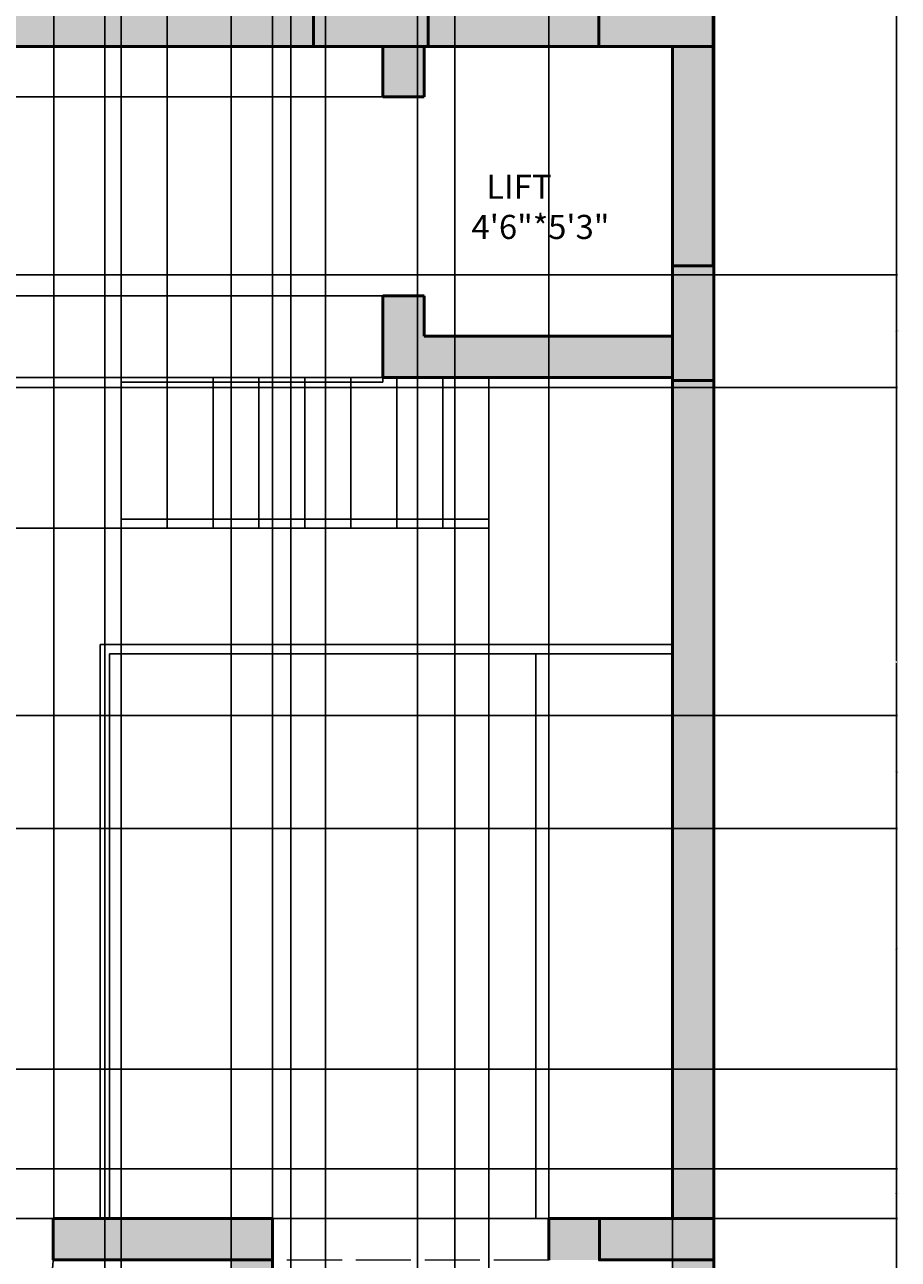
# Model space of a CAD drawing. Units: inches. Extents: x 2494 to 2908, y 1051 to 1885.
# Tile 5 of 7: x 2718 to 2908, y 1338 to 1607. Entities that reach past the tile are written whole.
import ezdxf

# ---------------------------------------------------------------- set-up
doc = ezdxf.new("R2010")
doc.units = ezdxf.units.IN
doc.linetypes.add('ACAD_ISO02W100', pattern=[15, 12, -3])
for name, color, linetype, lineweight in [('A-ANNO-DIMS', 2, 'Continuous', 18), ('A-AREA-IDEN', 130, 'Continuous', 18), ('A-COLS-PATT', 200, 'Continuous', 13), ('A-FLOR-HRAL', 140, 'Continuous', 25), ('A-FLOR-STRS', 7, 'Continuous', 25), ('A-WALL-OVHD', 140, 'ACAD_ISO02W100', 18), ('A-WALL-PATT', 140, 'Continuous', 13), ('COLUMN', 200, 'Continuous', 50), ('DOOR', 50, 'Continuous', 25), ('WALL', 140, 'Continuous', 50)]:
    doc.layers.add(name, color=color, linetype=linetype, lineweight=lineweight)
doc.styles.get("Standard").update_dxf_attribs({"font": 'arial.ttf'})
doc.dimstyles.get("Standard").update_dxf_attribs({"dimtxt": 0.18, "dimasz": 0.18, "dimexe": 0.18, "dimexo": 0.0625, "dimgap": 0.09, "dimtad": 0, "dimtih": 1, "dimtoh": 1, "dimdec": 4, "dimzin": 0, "dimdsep": 46, "dimtxsty": 'Standard', "dimcen": 0.09, "dimadec": 0, "dimazin": 0, "dimtfac": 1, "dimtdec": 4, "dimtofl": 0, "dimtmove": 0, "dimatfit": 3, "dimfxl": 1, "dimtolj": 1, "dimtzin": 0, "dimarcsym": 0})

# ---------------------------------------------------------------- blocks, each defined once
blk = doc.blocks.new('*U2')
for p, q in [((0, 0), (0, -6)), ((40, 0), (40, -6))]:
    blk.add_line(p, q)
blk.add_lwpolyline([(0, 0), (0, 40), (1.75, 40), (1.75, 0)], close=True)
blk.add_arc((0, 0), 40, 0, 90)
blk = doc.blocks.new('*D26')
at = {"layer": 'A-ANNO-DIMS', "color": 0, "lineweight": -2, "transparency": 16777216}
for p, q in [((2868.31, 1845.16), (2908.18, 1845.16)), ((2908, 1844.98), (2908, 1468.43)), ((2908, 1091.52), (2908, 1468.07)), ((2860.37, 1091.34), (2908.18, 1091.34))]:
    blk.add_line(p, q, dxfattribs=at)
at = {"layer": 'A-ANNO-DIMS', "color": 0, "lineweight": 100, "transparency": 16777216}
for points in [[(2907.97, 1844.98), (2908.03, 1844.98), (2908, 1845.16)], [(2907.97, 1091.52), (2908.03, 1091.52), (2908, 1091.34)]]:
    blk.add_solid(points, dxfattribs=at)
at = {"layer": 'Defpoints', "color": 0, "lineweight": 100, "transparency": 16777216}
for p in [(2868.25, 1845.16), (2908, 1845.16), (2860.3, 1091.34)]:
    blk.add_point(p, dxfattribs=at)
at = {"layer": 'A-ANNO-DIMS', "color": 0, "transparency": 16777216, "insert": (2908, 1468.25), "char_height": 0.18, "attachment_point": 5}
blk.add_mtext('\\A1;753.8', dxfattribs=at)
blk = doc.blocks.new('*D33')
at = {"layer": 'A-ANNO-DIMS', "color": 0, "lineweight": -2, "transparency": 16777216}
for p, q in [((2697.84, 1155.22), (2697.84, 1885.09)), ((2698.02, 1884.91), (2716.38, 1884.91)), ((2735.54, 1884.91), (2717.17, 1884.91)), ((2735.72, 1155.22), (2735.72, 1885.09))]:
    blk.add_line(p, q, dxfattribs=at)
at = {"layer": 'A-ANNO-DIMS', "color": 0, "lineweight": 100, "transparency": 16777216}
for points in [[(2698.02, 1884.94), (2698.02, 1884.88), (2697.84, 1884.91)], [(2735.54, 1884.94), (2735.54, 1884.88), (2735.72, 1884.91)]]:
    blk.add_solid(points, dxfattribs=at)
at = {"layer": 'Defpoints', "color": 0, "lineweight": 100, "transparency": 16777216}
for p in [(2735.72, 1884.91), (2697.84, 1155.16), (2735.72, 1155.16)]:
    blk.add_point(p, dxfattribs=at)
at = {"layer": 'A-ANNO-DIMS', "color": 0, "transparency": 16777216, "insert": (2716.78, 1884.91), "char_height": 0.18, "attachment_point": 5}
blk.add_mtext('\\A1;37.88', dxfattribs=at)
blk = doc.blocks.new('*D35')
at = {"layer": 'A-ANNO-DIMS', "color": 0, "lineweight": -2, "transparency": 16777216}
for p, q in [((2735.72, 1155.22), (2735.72, 1885.09)), ((2735.9, 1884.91), (2749.09, 1884.91)), ((2763.07, 1884.91), (2749.88, 1884.91)), ((2763.25, 1155.22), (2763.25, 1885.09))]:
    blk.add_line(p, q, dxfattribs=at)
at = {"layer": 'A-ANNO-DIMS', "color": 0, "lineweight": 100, "transparency": 16777216}
for points in [[(2735.9, 1884.94), (2735.9, 1884.88), (2735.72, 1884.91)], [(2763.07, 1884.94), (2763.07, 1884.88), (2763.25, 1884.91)]]:
    blk.add_solid(points, dxfattribs=at)
at = {"layer": 'Defpoints', "color": 0, "lineweight": 100, "transparency": 16777216}
for p in [(2763.25, 1884.91), (2735.72, 1155.16), (2763.25, 1155.16)]:
    blk.add_point(p, dxfattribs=at)
at = {"layer": 'A-ANNO-DIMS', "color": 0, "transparency": 16777216, "insert": (2749.49, 1884.91), "char_height": 0.18, "attachment_point": 5}
blk.add_mtext('\\A1;27.53', dxfattribs=at)
blk = doc.blocks.new('*D37')
at = {"layer": 'A-ANNO-DIMS', "color": 0, "lineweight": -2, "transparency": 16777216}
for p, q in [((2783.78, 1155.22), (2783.78, 1885.09)), ((2783.96, 1884.91), (2797.38, 1884.91)), ((2811.73, 1884.91), (2798.31, 1884.91)), ((2811.91, 1155.22), (2811.91, 1885.09))]:
    blk.add_line(p, q, dxfattribs=at)
at = {"layer": 'A-ANNO-DIMS', "color": 0, "lineweight": 100, "transparency": 16777216}
for points in [[(2783.96, 1884.94), (2783.96, 1884.88), (2783.78, 1884.91)], [(2811.73, 1884.94), (2811.73, 1884.88), (2811.91, 1884.91)]]:
    blk.add_solid(points, dxfattribs=at)
at = {"layer": 'Defpoints', "color": 0, "lineweight": 100, "transparency": 16777216}
for p in [(2811.91, 1884.91), (2783.78, 1155.16), (2811.91, 1155.16)]:
    blk.add_point(p, dxfattribs=at)
at = {"layer": 'A-ANNO-DIMS', "color": 0, "transparency": 16777216, "insert": (2797.85, 1884.91), "char_height": 0.18, "attachment_point": 5}
blk.add_mtext('\\A1;28.126', dxfattribs=at)
blk = doc.blocks.new('*D41')
at = {"layer": 'A-ANNO-DIMS', "color": 0, "lineweight": -2, "transparency": 16777216}
for p, q in [((2684.64, 1347.22), (2684.64, 1885.09)), ((2684.82, 1884.91), (2704.42, 1884.91)), ((2724.46, 1884.91), (2704.86, 1884.91)), ((2724.64, 1347.22), (2724.64, 1885.09))]:
    blk.add_line(p, q, dxfattribs=at)
at = {"layer": 'A-ANNO-DIMS', "color": 0, "lineweight": 100, "transparency": 16777216}
for points in [[(2684.82, 1884.94), (2684.82, 1884.88), (2684.64, 1884.91)], [(2724.46, 1884.94), (2724.46, 1884.88), (2724.64, 1884.91)]]:
    blk.add_solid(points, dxfattribs=at)
at = {"layer": 'Defpoints', "color": 0, "lineweight": 100, "transparency": 16777216}
for p in [(2724.64, 1884.91), (2684.64, 1347.16), (2724.64, 1347.16)]:
    blk.add_point(p, dxfattribs=at)
at = {"layer": 'A-ANNO-DIMS', "color": 0, "transparency": 16777216, "insert": (2704.64, 1884.91), "char_height": 0.18, "attachment_point": 5}
blk.add_mtext('\\A1;40', dxfattribs=at)
blk = doc.blocks.new('*D43')
at = {"layer": 'A-ANNO-DIMS', "color": 0, "lineweight": -2, "transparency": 16777216}
for p, q in [((2776.2, 1243.72), (2776.2, 1885.09)), ((2776.38, 1884.91), (2789.53, 1884.91)), ((2803.62, 1884.91), (2790.46, 1884.91)), ((2803.8, 1243.72), (2803.8, 1885.09))]:
    blk.add_line(p, q, dxfattribs=at)
at = {"layer": 'A-ANNO-DIMS', "color": 0, "lineweight": 100, "transparency": 16777216}
for points in [[(2776.38, 1884.94), (2776.38, 1884.88), (2776.2, 1884.91)], [(2803.62, 1884.94), (2803.62, 1884.88), (2803.8, 1884.91)]]:
    blk.add_solid(points, dxfattribs=at)
at = {"layer": 'Defpoints', "color": 0, "lineweight": 100, "transparency": 16777216}
for p in [(2803.8, 1884.91), (2776.2, 1243.66), (2803.8, 1243.66)]:
    blk.add_point(p, dxfattribs=at)
at = {"layer": 'A-ANNO-DIMS', "color": 0, "transparency": 16777216, "insert": (2790, 1884.91), "char_height": 0.18, "attachment_point": 5}
blk.add_mtext('\\A1;27.604', dxfattribs=at)
blk = doc.blocks.new('*D44')
at = {"layer": 'A-ANNO-DIMS', "color": 0, "lineweight": -2, "transparency": 16777216}
for p, q in [((2772.25, 1347.22), (2772.25, 1885.09)), ((2772.43, 1884.91), (2801.99, 1884.91)), ((2832.17, 1884.91), (2802.61, 1884.91)), ((2832.35, 1347.22), (2832.35, 1885.09))]:
    blk.add_line(p, q, dxfattribs=at)
at = {"layer": 'A-ANNO-DIMS', "color": 0, "lineweight": 100, "transparency": 16777216}
for points in [[(2772.43, 1884.94), (2772.43, 1884.88), (2772.25, 1884.91)], [(2832.17, 1884.94), (2832.17, 1884.88), (2832.35, 1884.91)]]:
    blk.add_solid(points, dxfattribs=at)
at = {"layer": 'Defpoints', "color": 0, "lineweight": 100, "transparency": 16777216}
for p in [(2832.35, 1884.91), (2772.25, 1347.16), (2832.35, 1347.16)]:
    blk.add_point(p, dxfattribs=at)
at = {"layer": 'A-ANNO-DIMS', "color": 0, "transparency": 16777216, "insert": (2802.3, 1884.91), "char_height": 0.18, "attachment_point": 5}
blk.add_mtext('\\A1;60.1', dxfattribs=at)
blk = doc.blocks.new('*D46')
at = {"layer": 'A-ANNO-DIMS', "color": 0, "lineweight": -2, "transparency": 16777216}
for p, q in [((2674.81, 1432.05), (2908.18, 1432.05)), ((2908, 1431.87), (2908, 1406.05)), ((2908, 1379.87), (2908, 1405.69)), ((2674.81, 1379.69), (2908.18, 1379.69))]:
    blk.add_line(p, q, dxfattribs=at)
at = {"layer": 'A-ANNO-DIMS', "color": 0, "lineweight": 100, "transparency": 16777216}
for points in [[(2907.97, 1431.87), (2908.03, 1431.87), (2908, 1432.05)], [(2907.97, 1379.87), (2908.03, 1379.87), (2908, 1379.69)]]:
    blk.add_solid(points, dxfattribs=at)
at = {"layer": 'Defpoints', "color": 0, "lineweight": 100, "transparency": 16777216}
for p in [(2674.75, 1432.05), (2908, 1432.05), (2674.75, 1379.69)]:
    blk.add_point(p, dxfattribs=at)
at = {"layer": 'A-ANNO-DIMS', "color": 0, "transparency": 16777216, "insert": (2908, 1405.87), "char_height": 0.18, "attachment_point": 5}
blk.add_mtext('\\A1;52.36', dxfattribs=at)
blk = doc.blocks.new('*D47')
at = {"layer": 'A-ANNO-DIMS', "color": 0, "lineweight": -2, "transparency": 16777216}
for p, q in [((2674.81, 1456.66), (2908.18, 1456.66)), ((2908, 1456.48), (2908, 1444.53)), ((2908, 1432.23), (2908, 1444.17)), ((2674.81, 1432.05), (2908.18, 1432.05))]:
    blk.add_line(p, q, dxfattribs=at)
at = {"layer": 'A-ANNO-DIMS', "color": 0, "lineweight": 100, "transparency": 16777216}
for points in [[(2907.97, 1456.48), (2908.03, 1456.48), (2908, 1456.66)], [(2907.97, 1432.23), (2908.03, 1432.23), (2908, 1432.05)]]:
    blk.add_solid(points, dxfattribs=at)
at = {"layer": 'Defpoints', "color": 0, "lineweight": 100, "transparency": 16777216}
for p in [(2674.75, 1456.66), (2908, 1456.66), (2674.75, 1432.05)]:
    blk.add_point(p, dxfattribs=at)
at = {"layer": 'A-ANNO-DIMS', "color": 0, "transparency": 16777216, "insert": (2908, 1444.35), "char_height": 0.18, "attachment_point": 5}
blk.add_mtext('\\A1;24.606', dxfattribs=at)
blk = doc.blocks.new('*D52')
at = {"layer": 'A-ANNO-DIMS', "color": 0, "lineweight": -2, "transparency": 16777216}
for p, q in [((2649.94, 1358.01), (2908.18, 1358.01)), ((2908, 1357.83), (2908, 1352.76)), ((2908, 1347.34), (2908, 1352.4)), ((2670.31, 1347.16), (2908.18, 1347.16))]:
    blk.add_line(p, q, dxfattribs=at)
at = {"layer": 'A-ANNO-DIMS', "color": 0, "lineweight": 100, "transparency": 16777216}
for points in [[(2907.97, 1357.83), (2908.03, 1357.83), (2908, 1358.01)], [(2907.97, 1347.34), (2908.03, 1347.34), (2908, 1347.16)]]:
    blk.add_solid(points, dxfattribs=at)
at = {"layer": 'Defpoints', "color": 0, "lineweight": 100, "transparency": 16777216}
for p in [(2649.88, 1358.01), (2908, 1358.01), (2670.25, 1347.16)]:
    blk.add_point(p, dxfattribs=at)
at = {"layer": 'A-ANNO-DIMS', "color": 0, "transparency": 16777216, "insert": (2908, 1352.58), "char_height": 0.18, "attachment_point": 5}
blk.add_mtext('\\A1;10.852', dxfattribs=at)
blk = doc.blocks.new('*D53')
at = {"layer": 'A-ANNO-DIMS', "color": 0, "lineweight": -2, "transparency": 16777216}
for p, q in [((2739.28, 1497.29), (2739.28, 1051.41)), ((2819.28, 1497.29), (2819.28, 1051.41)), ((2739.46, 1051.59), (2779.06, 1051.59)), ((2819.1, 1051.59), (2779.5, 1051.59))]:
    blk.add_line(p, q, dxfattribs=at)
at = {"layer": 'A-ANNO-DIMS', "color": 0, "lineweight": 100, "transparency": 16777216}
for points in [[(2739.46, 1051.62), (2739.46, 1051.56), (2739.28, 1051.59)], [(2819.1, 1051.62), (2819.1, 1051.56), (2819.28, 1051.59)]]:
    blk.add_solid(points, dxfattribs=at)
at = {"layer": 'Defpoints', "color": 0, "lineweight": 100, "transparency": 16777216}
for p in [(2739.28, 1497.36), (2819.28, 1497.36), (2819.28, 1051.59)]:
    blk.add_point(p, dxfattribs=at)
at = {"layer": 'A-ANNO-DIMS', "color": 0, "transparency": 16777216, "insert": (2779.28, 1051.59), "char_height": 0.18, "attachment_point": 5}
blk.add_mtext('\\A1;80', dxfattribs=at)
blk = doc.blocks.new('*D54')
at = {"layer": 'A-ANNO-DIMS', "color": 0, "lineweight": -2, "transparency": 16777216}
for p, q in [((2739.21, 1530.16), (2494.47, 1530.16)), ((2494.65, 1529.98), (2494.65, 1513.94)), ((2494.65, 1497.54), (2494.65, 1513.57)), ((2739.21, 1497.36), (2494.47, 1497.36))]:
    blk.add_line(p, q, dxfattribs=at)
at = {"layer": 'A-ANNO-DIMS', "color": 0, "lineweight": 100, "transparency": 16777216}
for points in [[(2494.62, 1529.98), (2494.68, 1529.98), (2494.65, 1530.16)], [(2494.62, 1497.54), (2494.68, 1497.54), (2494.65, 1497.36)]]:
    blk.add_solid(points, dxfattribs=at)
at = {"layer": 'Defpoints', "color": 0, "lineweight": 100, "transparency": 16777216}
for p in [(2494.65, 1530.16), (2739.28, 1530.16), (2739.28, 1497.36)]:
    blk.add_point(p, dxfattribs=at)
at = {"layer": 'A-ANNO-DIMS', "color": 0, "transparency": 16777216, "insert": (2494.65, 1513.76), "char_height": 0.18, "attachment_point": 5}
blk.add_mtext('\\A1;32.8', dxfattribs=at)
blk = doc.blocks.new('*D55')
at = {"layer": 'A-ANNO-DIMS', "color": 0, "lineweight": -2, "transparency": 16777216}
for p, q in [((2739.28, 1530.22), (2739.28, 1885.09)), ((2739.46, 1884.91), (2744.07, 1884.91)), ((2749.1, 1884.91), (2744.49, 1884.91)), ((2749.28, 1530.22), (2749.28, 1885.09))]:
    blk.add_line(p, q, dxfattribs=at)
at = {"layer": 'A-ANNO-DIMS', "color": 0, "lineweight": 100, "transparency": 16777216}
for points in [[(2739.46, 1884.94), (2739.46, 1884.88), (2739.28, 1884.91)], [(2749.1, 1884.94), (2749.1, 1884.88), (2749.28, 1884.91)]]:
    blk.add_solid(points, dxfattribs=at)
at = {"layer": 'Defpoints', "color": 0, "lineweight": 100, "transparency": 16777216}
for p in [(2749.28, 1884.91), (2739.28, 1530.16), (2749.28, 1530.16)]:
    blk.add_point(p, dxfattribs=at)
at = {"layer": 'A-ANNO-DIMS', "color": 0, "transparency": 16777216, "insert": (2744.28, 1884.91), "char_height": 0.18, "attachment_point": 5}
blk.add_mtext('\\A1;10', dxfattribs=at)
blk = doc.blocks.new('*D56')
at = {"layer": 'A-ANNO-DIMS', "color": 0, "lineweight": -2, "transparency": 16777216}
for p, q in [((2819.28, 1530.09), (2819.28, 1051.41)), ((2859.25, 1530.09), (2859.25, 1051.41)), ((2819.46, 1051.59), (2838.8, 1051.59)), ((2859.07, 1051.59), (2839.73, 1051.59))]:
    blk.add_line(p, q, dxfattribs=at)
at = {"layer": 'A-ANNO-DIMS', "color": 0, "lineweight": 100, "transparency": 16777216}
for points in [[(2819.46, 1051.62), (2819.46, 1051.56), (2819.28, 1051.59)], [(2859.07, 1051.62), (2859.07, 1051.56), (2859.25, 1051.59)]]:
    blk.add_solid(points, dxfattribs=at)
at = {"layer": 'Defpoints', "color": 0, "lineweight": 100, "transparency": 16777216}
for p in [(2819.28, 1530.16), (2859.25, 1530.16), (2859.25, 1051.59)]:
    blk.add_point(p, dxfattribs=at)
at = {"layer": 'A-ANNO-DIMS', "color": 0, "transparency": 16777216, "insert": (2839.26, 1051.59), "char_height": 0.18, "attachment_point": 5}
blk.add_mtext('\\A1;39.975', dxfattribs=at)
blk = doc.blocks.new('*D57')
at = {"layer": 'A-ANNO-DIMS', "color": 0, "lineweight": -2, "transparency": 16777216}
for p, q in [((2796.19, 1591.24), (2494.47, 1591.24)), ((2494.65, 1591.06), (2494.65, 1569.76)), ((2494.65, 1548.09), (2494.65, 1569.39)), ((2796.19, 1547.91), (2494.47, 1547.91))]:
    blk.add_line(p, q, dxfattribs=at)
at = {"layer": 'A-ANNO-DIMS', "color": 0, "lineweight": 100, "transparency": 16777216}
for points in [[(2494.62, 1591.06), (2494.68, 1591.06), (2494.65, 1591.24)], [(2494.62, 1548.09), (2494.68, 1548.09), (2494.65, 1547.91)]]:
    blk.add_solid(points, dxfattribs=at)
at = {"layer": 'Defpoints', "color": 0, "lineweight": 100, "transparency": 16777216}
for p in [(2494.65, 1591.24), (2796.25, 1591.24), (2796.25, 1547.91)]:
    blk.add_point(p, dxfattribs=at)
at = {"layer": 'A-ANNO-DIMS', "color": 0, "transparency": 16777216, "insert": (2494.65, 1569.57), "char_height": 0.18, "attachment_point": 5}
blk.add_mtext('\\A1;43.324', dxfattribs=at)
blk = doc.blocks.new('*D58')
at = {"layer": 'A-ANNO-DIMS', "color": 0, "lineweight": -2, "transparency": 16777216}
for p, q in [((2796.19, 1602.16), (2494.47, 1602.16)), ((2494.65, 1601.98), (2494.65, 1596.88)), ((2494.65, 1591.42), (2494.65, 1596.51)), ((2796.19, 1591.24), (2494.47, 1591.24))]:
    blk.add_line(p, q, dxfattribs=at)
at = {"layer": 'A-ANNO-DIMS', "color": 0, "lineweight": 100, "transparency": 16777216}
for points in [[(2494.62, 1601.98), (2494.68, 1601.98), (2494.65, 1602.16)], [(2494.62, 1591.42), (2494.68, 1591.42), (2494.65, 1591.24)]]:
    blk.add_solid(points, dxfattribs=at)
at = {"layer": 'Defpoints', "color": 0, "lineweight": 100, "transparency": 16777216}
for p in [(2494.65, 1602.16), (2796.25, 1602.16), (2796.25, 1591.24)]:
    blk.add_point(p, dxfattribs=at)
at = {"layer": 'A-ANNO-DIMS', "color": 0, "transparency": 16777216, "insert": (2494.65, 1596.7), "char_height": 0.18, "attachment_point": 5}
blk.add_mtext('\\A1;10.92', dxfattribs=at)
blk = doc.blocks.new('*D59')
at = {"layer": 'A-ANNO-DIMS', "color": 0, "lineweight": -2, "transparency": 16777216}
for p, q in [((2859.25, 1530.09), (2859.25, 1051.41)), ((2868.25, 1529.48), (2868.25, 1051.41)), ((2859.43, 1051.59), (2863.6, 1051.59)), ((2868.07, 1051.59), (2863.9, 1051.59))]:
    blk.add_line(p, q, dxfattribs=at)
at = {"layer": 'A-ANNO-DIMS', "color": 0, "lineweight": 100, "transparency": 16777216}
for points in [[(2859.43, 1051.62), (2859.43, 1051.56), (2859.25, 1051.59)], [(2868.07, 1051.62), (2868.07, 1051.56), (2868.25, 1051.59)]]:
    blk.add_solid(points, dxfattribs=at)
at = {"layer": 'Defpoints', "color": 0, "lineweight": 100, "transparency": 16777216}
for p in [(2859.25, 1530.16), (2868.25, 1529.54), (2868.25, 1051.59)]:
    blk.add_point(p, dxfattribs=at)
at = {"layer": 'A-ANNO-DIMS', "color": 0, "transparency": 16777216, "insert": (2863.75, 1051.59), "char_height": 0.18, "attachment_point": 5}
blk.add_mtext('\\A1;9', dxfattribs=at)
blk = doc.blocks.new('*D63')
at = {"layer": 'A-ANNO-DIMS', "color": 0, "lineweight": -2, "transparency": 16777216}
for p, q in [((2628.75, 1552.53), (2908.18, 1552.53)), ((2908, 1552.35), (2908, 1540.45)), ((2908, 1528.19), (2908, 1540.09)), ((2628.75, 1528.01), (2908.18, 1528.01))]:
    blk.add_line(p, q, dxfattribs=at)
at = {"layer": 'A-ANNO-DIMS', "color": 0, "lineweight": 100, "transparency": 16777216}
for points in [[(2907.97, 1552.35), (2908.03, 1552.35), (2908, 1552.53)], [(2907.97, 1528.19), (2908.03, 1528.19), (2908, 1528.01)]]:
    blk.add_solid(points, dxfattribs=at)
at = {"layer": 'Defpoints', "color": 0, "lineweight": 100, "transparency": 16777216}
for p in [(2628.68, 1552.53), (2908, 1552.53), (2628.68, 1528.01)]:
    blk.add_point(p, dxfattribs=at)
at = {"layer": 'A-ANNO-DIMS', "color": 0, "transparency": 16777216, "insert": (2908, 1540.27), "char_height": 0.18, "attachment_point": 5}
blk.add_mtext('\\A1;24.523', dxfattribs=at)

msp = doc.modelspace()

# ---------------------------------------------------------------- hatches: boundary and pattern name
at = {"layer": 'A-COLS-PATT'}
h = msp.add_hatch(color=256, dxfattribs=at)
h.dxf.hatch_style = 1
h.paths.add_polyline_path([(2584.1612, 1845.1561), (2559.2517, 1845.1561), (2559.2517, 1836.1561), (2584.1612, 1836.1561)])
h.paths.add_polyline_path([(2720.7462, 1845.1561), (2695.8368, 1845.1561), (2695.8368, 1836.1561), (2720.7462, 1836.1561)])
h.paths.add_polyline_path([(2868.2517, 1845.1561), (2843.3423, 1845.1561), (2843.3423, 1836.1561), (2868.2517, 1836.1561)])
h.paths.add_polyline_path([(2568.2517, 1728.1561), (2559.2517, 1728.1561), (2559.2517, 1703.2467), (2568.2517, 1703.2467)])
h.paths.add_polyline_path([(2568.2517, 1564.0885), (2559.2517, 1564.0885), (2559.2517, 1539.1791), (2568.2517, 1539.1791)])
h.paths.add_polyline_path([(2868.2517, 1554.4528), (2859.2517, 1554.4528), (2859.2517, 1529.5434), (2868.2517, 1529.5434)])
h.paths.add_polyline_path([(2806.0841, 1611.1561), (2781.1746, 1611.1561), (2781.1746, 1602.1561), (2806.0841, 1602.1561)])
h.paths.add_polyline_path([(2868.0971, 1611.1561), (2843.1877, 1611.1561), (2843.1877, 1602.1561), (2868.0971, 1602.1561)])
h.paths.add_polyline_path([(2584.1612, 1347.1561), (2559.2517, 1347.1561), (2559.2517, 1338.1561), (2584.1612, 1338.1561)])
h.paths.add_polyline_path([(2868.2517, 1347.1561), (2843.3423, 1347.1561), (2843.3423, 1338.1561), (2868.2517, 1338.1561)])
h.paths.add_polyline_path([(2568.2517, 1180.0656), (2559.2517, 1180.0656), (2559.2517, 1155.1561), (2568.2517, 1155.1561)])
h.paths.add_polyline_path([(2584.1612, 1155.1561), (2559.2517, 1155.1561), (2559.2517, 1146.1561), (2584.1612, 1146.1561)])
h.paths.add_polyline_path([(2868.2517, 1155.1561), (2843.3423, 1155.1561), (2843.3423, 1146.1561), (2868.2517, 1146.1561)])
h.paths.add_polyline_path([(2868.2517, 1180.0656), (2859.2517, 1180.0656), (2859.2517, 1155.1561), (2868.2517, 1155.1561)])
at = {"layer": 'A-WALL-PATT'}
h = msp.add_hatch(color=256, dxfattribs=at)
h.dxf.hatch_style = 1
h.paths.add_polyline_path([(2609.6092, 1845.1561), (2584.1612, 1845.1561), (2584.1612, 1836.1561), (2609.6092, 1836.1561)])
h.paths.add_polyline_path([(2695.8368, 1845.1561), (2672.7564, 1845.1561), (2672.7564, 1836.1561), (2695.8368, 1836.1561)])
h.paths.add_polyline_path([(2767.7517, 1845.1561), (2720.7462, 1845.1561), (2720.7462, 1836.1561), (2763.2517, 1836.1561), (2763.2517, 1808.7615), (2767.7517, 1808.7615)])
h.paths.add_polyline_path([(2843.3423, 1845.1561), (2767.7517, 1845.1561), (2767.7517, 1836.1561), (2843.3423, 1836.1561)])
h.paths.add_polyline_path([(2568.2517, 1836.1561), (2559.2517, 1836.1561), (2559.2517, 1728.1561), (2568.2517, 1728.1561)])
h.paths.add_polyline_path([(2568.2517, 1703.2467), (2559.2517, 1703.2467), (2559.2517, 1611.1561), (2568.2517, 1611.1561)])
h.paths.add_polyline_path([(2843.1877, 1611.1561), (2819.0012, 1611.1561), (2806.0841, 1611.1561), (2806.0841, 1602.1561), (2843.1877, 1602.1561)])
h.paths.add_polyline_path([(2805.2517, 1602.1561), (2796.2517, 1602.1561), (2796.2517, 1591.2367), (2805.2517, 1591.2367)])
h = msp.add_hatch(color=256, dxfattribs=at)
h.dxf.hatch_style = 1
h.paths.add_polyline_path([(2868.2517, 1836.1561), (2859.2517, 1836.1561), (2859.2517, 1611.1561), (2868.2517, 1611.1561)])
h.paths.add_polyline_path([(2715.2517, 1611.1561), (2655.4916, 1611.1561), (2655.4916, 1606.6561), (2715.2517, 1606.6561)])
h.paths.add_polyline_path([(2781.1746, 1611.1561), (2776.9029, 1611.1561), (2715.2517, 1611.1561), (2715.2517, 1606.6561), (2715.2517, 1602.1561), (2781.1746, 1602.1561)])
h.paths.add_polyline_path([(2868.0971, 1602.1561), (2859.2517, 1602.1561), (2859.2517, 1554.4528), (2868.0971, 1554.4528)])
h.paths.add_polyline_path([(2868.2517, 1529.5434), (2859.2517, 1529.5434), (2859.2517, 1347.1561), (2868.2517, 1347.1561)])
h.paths.add_polyline_path([(2868.2517, 1338.1561), (2859.2517, 1338.1561), (2859.2517, 1243.6561), (2868.2517, 1243.6561)])
h.paths.add_polyline_path([(2568.2517, 1338.1561), (2559.2517, 1338.1561), (2559.2517, 1180.0656), (2568.2517, 1180.0656)])
h.paths.add_polyline_path([(2735.7191, 1155.1561), (2697.838, 1155.1561), (2697.838, 1146.1561), (2735.7191, 1146.1561), (2735.7191, 1151.0155)])
h = msp.add_hatch(color=256, dxfattribs=at)
h.dxf.hatch_style = 1
h.paths.add_polyline_path([(2805.2517, 1547.9123), (2796.2517, 1547.9123), (2796.2517, 1530.1561), (2859.2517, 1530.1561), (2859.2517, 1539.1561), (2805.2517, 1539.1561)])
h.paths.add_polyline_path([(2568.2517, 1606.6561), (2615.4916, 1606.6561), (2615.4916, 1611.1561), (2559.2517, 1611.1561), (2559.2517, 1564.0885), (2568.2517, 1564.0885)])
h.paths.add_polyline_path([(2568.2517, 1539.1791), (2559.2517, 1539.1791), (2559.2517, 1456.6561), (2534.4016, 1456.6561), (2534.4016, 1338.1561), (2559.2517, 1338.1561), (2559.2517, 1342.6561), (2543.4016, 1342.6561), (2543.4016, 1452.1561), (2559.2517, 1452.1561), (2568.2517, 1452.1561), (2674.7517, 1452.1561), (2674.7517, 1456.6561), (2568.2517, 1456.6561)])
h.paths.add_polyline_path([(2684.6403, 1347.1561), (2674.7517, 1347.1561), (2584.1612, 1347.1561), (2584.1612, 1338.1561), (2684.6403, 1338.1561), (2684.6403, 1341.1561)])
h.paths.add_polyline_path([(2843.3423, 1347.1561), (2832.3482, 1347.1561), (2832.3482, 1338.1485), (2843.3423, 1338.1485)])
h.paths.add_polyline_path([(2634.6908, 1155.1561), (2584.1612, 1155.1561), (2584.1612, 1146.1561), (2634.6908, 1146.1561)])
h.paths.add_polyline_path([(2783.7833, 1155.1561), (2772.2517, 1155.1561), (2772.2517, 1146.1561), (2783.7833, 1146.1561)])
h.paths.add_polyline_path([(2843.3423, 1155.1561), (2819.0012, 1155.1561), (2811.9091, 1155.1561), (2811.9091, 1146.1561), (2843.3423, 1146.1561)])
h.paths.add_polyline_path([(2868.2517, 1243.6561), (2859.2517, 1243.6561), (2859.2517, 1239.1561), (2859.2517, 1180.0656), (2868.2517, 1180.0656)])
h = msp.add_hatch(color=256, dxfattribs=at)
h.dxf.hatch_style = 1
h.paths.add_polyline_path([(2772.2517, 1338.1561), (2763.2517, 1338.1561), (2763.2517, 1146.1561), (2772.2517, 1146.1561)])
h.paths.add_polyline_path([(2772.2517, 1347.1561), (2724.6403, 1347.1561), (2724.6403, 1341.1561, -0.01876983), (2724.5277, 1338.1561), (2772.2517, 1338.1561)])
h.paths.add_polyline_path([(2808.4276, 1199.3021), (2836.8916, 1199.3021), (2836.8916, 1218.8855), (2808.4276, 1218.8855)], flags=9)
h.paths.add_polyline_path([(2797.835, 1285.0138), (2820.947, 1285.0138), (2820.947, 1304.5973), (2797.835, 1304.5973)], flags=9)

# ---------------------------------------------------------------- linework, layer by layer
at = {"layer": 'A-FLOR-HRAL'}
for p, q in [((2734.7517, 1456.6561), (2734.7517, 1472.0627)), ((2734.7517, 1472.0627), (2859.2517, 1472.0627)), ((2736.7517, 1470.0627), (2859.2517, 1470.0627)), ((2736.7517, 1456.6561), (2736.7517, 1470.0627)), ((2829.5289, 1470.0627), (2829.5289, 1347.1561)), ((2734.7517, 1347.1561), (2734.7517, 1456.6561)), ((2736.7517, 1347.1561), (2736.7517, 1456.6561))]:
    msp.add_line(p, q, dxfattribs=at)
at = {"layer": 'A-FLOR-STRS'}
for p, q in [((2796.2517, 1530.1561), (2739.2763, 1530.1561)), ((2739.2763, 1530.1561), (2739.2763, 1497.3573)), ((2796.2517, 1529.1561), (2739.2763, 1529.1561)), ((2749.2763, 1530.1561), (2749.2763, 1497.3573)), ((2759.2763, 1530.1561), (2759.2763, 1497.3573)), ((2769.2763, 1530.1561), (2769.2763, 1497.3573)), ((2779.2763, 1530.1561), (2779.2763, 1497.3573)), ((2789.2763, 1530.1561), (2789.2763, 1497.3573)), ((2796.2517, 1529.1561), (2796.2517, 1530.9723)), ((2799.2763, 1530.1561), (2799.2763, 1497.3573)), ((2809.2763, 1530.1561), (2809.2763, 1497.3573)), ((2819.2763, 1530.1561), (2819.2763, 1497.3573)), ((2819.2763, 1499.3573), (2739.2763, 1499.3573)), ((2819.2763, 1497.3573), (2739.2763, 1497.3573)), ((2819.2763, 1497.3573), (2739.2763, 1497.3573))]:
    msp.add_line(p, q, dxfattribs=at)
at = {"layer": 'A-WALL-OVHD'}
msp.add_lwpolyline([(2772.2517, 1347.1561), (2832.3482, 1347.1561), (2832.3482, 1338.1485), (2772.2517, 1338.1485)], close=True, dxfattribs=at)
at = {"layer": 'COLUMN'}
for points in [[(2781.1746, 1611.1561), (2806.0841, 1611.1561), (2806.0841, 1602.1561), (2781.1746, 1602.1561)], [(2843.1877, 1611.1561), (2868.0971, 1611.1561), (2868.0971, 1602.1561), (2843.1877, 1602.1561)], [(2868.2517, 1554.4528), (2868.2517, 1529.5434), (2859.2517, 1529.5434), (2859.2517, 1554.4528)], [(2843.3423, 1347.1561), (2868.2517, 1347.1561), (2868.2517, 1338.1561), (2843.3423, 1338.1561)]]:
    msp.add_lwpolyline(points, close=True, dxfattribs=at)
at = {"layer": 'WALL'}
for p, q in [((2868.2517, 1347.1561), (2868.2517, 1611.1561)), ((2719.7517, 1602.1561), (2715.2517, 1602.1561)), ((2859.2517, 1602.1561), (2719.7517, 1602.1561)), ((2796.2517, 1591.2367), (2796.2517, 1602.1561)), ((2805.2517, 1591.2367), (2805.2517, 1602.1561)), ((2859.2517, 1347.1561), (2859.2517, 1602.1561)), ((2859.2517, 1602.1561), (2859.2517, 1539.1561)), ((2796.2517, 1530.1561), (2796.2517, 1547.9123)), ((2805.2517, 1539.1561), (2805.2517, 1547.9123)), ((2859.2517, 1539.1561), (2805.2517, 1539.1561)), ((2859.2517, 1530.1561), (2796.2517, 1530.1561)), ((2772.2517, 1347.1561), (2724.6403, 1347.1561)), ((2724.6403, 1347.1561), (2734.7517, 1347.1561)), ((2772.2517, 1146.1561), (2772.2517, 1347.1561)), ((2832.3482, 1347.1561), (2868.2517, 1347.1561)), ((2868.2517, 1243.6561), (2868.2517, 1347.1561))]:
    msp.add_line(p, q, dxfattribs=at)
for points in [[(2715.2517, 1602.1561), (2781.1746, 1602.1561), (2781.1746, 1611.1561), (2715.2517, 1611.1561)], [(2859.2517, 1554.4528), (2868.0971, 1554.4528), (2868.0971, 1602.1561), (2859.2517, 1602.1561)], [(2859.2517, 1347.1561), (2868.2517, 1347.1561), (2868.2517, 1529.5434), (2859.2517, 1529.5434)], [(2724.5277, 1338.1561), (2772.2517, 1338.1561), (2772.2517, 1347.1561), (2724.5277, 1347.1561)]]:
    msp.add_lwpolyline(points, close=True, dxfattribs=at)
for points in [[(2796.2517, 1591.2367), (2805.2517, 1591.2367)], [(2805.2517, 1547.9123), (2796.2517, 1547.9123)], [(2772.2517, 1347.1561), (2772.2517, 1338.1485)], [(2832.3482, 1338.1485), (2832.3482, 1347.1561)]]:
    msp.add_lwpolyline(points, dxfattribs=at)

# ---------------------------------------------------------------- block references
at = {"layer": 'DOOR', "xscale": -1, "rotation": 180}
msp.add_blockref('*U2', (2684.6403, 1341.1561), dxfattribs=at)

# ---------------------------------------------------------------- texts
at = {"layer": 'A-AREA-IDEN', "insert": (2815.5132, 1574.2943), "char_height": 5.24818, "attachment_point": 1}
msp.add_mtext_dynamic_manual_height_columns('  LIFT\\P4\'6"*5\'3"', width=250.978097, gutter_width=26.2409, heights=[0], dxfattribs=at)

# ---------------------------------------------------------------- dimensions: what is measured, and where the dimension line sits
at = {"layer": 'A-ANNO-DIMS'}
for base, p1, p2, override, picture, middle in [((2724.6403, 1884.9061), (2684.6403, 1347.1561), (2724.6403, 1347.1561), {"dimdec": 0, "dimlfac": 1, "dimrnd": 0, "dimzin": 0, "dimdsep": 46, "dimlunit": 2}, '*D41', (2704.6403, 1884.9061)), ((2735.7191, 1884.9061), (2697.838, 1155.1561), (2735.7191, 1155.1561), {"dimdec": 2, "dimlfac": 1, "dimrnd": 0, "dimzin": 0, "dimdsep": 46, "dimlunit": 2}, '*D33', (2716.7785, 1884.9061)), ((2763.2517, 1884.9061), (2735.7191, 1155.1561), (2763.2517, 1155.1561), {"dimdec": 2, "dimlfac": 1, "dimrnd": 0, "dimzin": 0, "dimdsep": 46, "dimlunit": 2}, '*D35', (2749.4854, 1884.9061)), ((2749.2763, 1884.9061), (2739.2763, 1530.1561), (2749.2763, 1530.1561), {"dimdec": 0, "dimlfac": 1, "dimrnd": 0, "dimzin": 0, "dimdsep": 46, "dimlunit": 2}, '*D55', (2744.2763, 1884.9061)), ((2832.3482, 1884.9061), (2772.2517, 1347.1561), (2832.3482, 1347.1561), {"dimdec": 1, "dimlfac": 1, "dimrnd": 0, "dimzin": 0, "dimdsep": 46, "dimlunit": 2}, '*D44', (2802.3, 1884.9061)), ((2803.8003, 1884.9061), (2776.196, 1243.6561), (2803.8003, 1243.6561), {"dimdec": 3, "dimlfac": 1, "dimrnd": 0, "dimzin": 0, "dimdsep": 46, "dimlunit": 2}, '*D43', (2789.9982, 1884.9061)), ((2811.9091, 1884.9061), (2783.7833, 1155.1561), (2811.9091, 1155.1561), {"dimdec": 3, "dimlfac": 1, "dimrnd": 0, "dimzin": 0, "dimdsep": 46, "dimlunit": 2}, '*D37', (2797.8462, 1884.9061)), ((2859.2517, 1051.5937), (2819.2763, 1530.1561), (2859.2517, 1530.1561), {"dimdec": 3, "dimlfac": 1, "dimrnd": 0, "dimzin": 0, "dimdsep": 46, "dimlunit": 2}, '*D56', (2839.264, 1051.5937)), ((2868.2517, 1051.5937), (2859.2517, 1530.1561), (2868.2517, 1529.5434), {"dimdec": 0, "dimlfac": 1, "dimrnd": 0, "dimzin": 0, "dimdsep": 46, "dimlunit": 2}, '*D59', (2863.7517, 1051.5937)), ((2819.2763, 1051.5937), (2739.2763, 1497.3573), (2819.2763, 1497.3573), {"dimdec": 0, "dimlfac": 1, "dimrnd": 0, "dimzin": 0, "dimdsep": 46, "dimlunit": 2}, '*D53', (2779.2763, 1051.5937))]:
    dim = msp.add_linear_dim(base=base, p1=p1, p2=p2, dimstyle='Standard', override=override, dxfattribs=at)
    dim.commit()
    dim.dimension.update_dxf_attribs({"geometry": picture, "text_midpoint": middle})
for base, p1, p2, override, picture, middle in [((2908.0017, 1845.1561), (2860.3038, 1091.3437), (2868.2517, 1845.1561), {"dimdec": 1, "dimlfac": 1, "dimrnd": 0, "dimzin": 0, "dimdsep": 46, "dimlunit": 2}, '*D26', (2908.0017, 1468.2499)), ((2494.6516, 1602.1561), (2796.2517, 1591.2367), (2796.2517, 1602.1561), {"dimdec": 2, "dimlfac": 1, "dimrnd": 0, "dimzin": 0, "dimdsep": 46, "dimlunit": 2}, '*D58', (2494.6516, 1596.6964)), ((2494.6516, 1591.2367), (2796.2517, 1547.9123), (2796.2517, 1591.2367), {"dimdec": 3, "dimlfac": 1, "dimrnd": 0, "dimzin": 0, "dimdsep": 46, "dimlunit": 2}, '*D57', (2494.6516, 1569.5745)), ((2908.0017, 1552.5335), (2628.6843, 1528.0102), (2628.6843, 1552.5335), {"dimdec": 3, "dimlfac": 1, "dimrnd": 0, "dimzin": 0, "dimdsep": 46, "dimlunit": 2}, '*D63', (2908.0017, 1540.2719)), ((2494.6516, 1530.1561), (2739.2763, 1497.3573), (2739.2763, 1530.1561), {"dimdec": 1, "dimlfac": 1, "dimrnd": 0, "dimzin": 0, "dimdsep": 46, "dimlunit": 2}, '*D54', (2494.6516, 1513.7567)), ((2908.0017, 1456.6561), (2674.7517, 1432.0498), (2674.7517, 1456.6561), {"dimdec": 3, "dimlfac": 1, "dimrnd": 0, "dimzin": 0, "dimdsep": 46, "dimlunit": 2}, '*D47', (2908.0017, 1444.353)), ((2908.0017, 1432.0498), (2674.7517, 1379.6865), (2674.7517, 1432.0498), {"dimdec": 2, "dimlfac": 1, "dimrnd": 0, "dimzin": 0, "dimdsep": 46, "dimlunit": 2}, '*D46', (2908.0017, 1405.8682)), ((2908.0017, 1358.0085), (2670.2517, 1347.1561), (2649.877, 1358.0085), {"dimdec": 3, "dimlfac": 1, "dimrnd": 0, "dimzin": 0, "dimdsep": 46, "dimlunit": 2}, '*D52', (2908.0017, 1352.5823))]:
    dim = msp.add_linear_dim(base=base, p1=p1, p2=p2, angle=90, dimstyle='Standard', override=override, dxfattribs=at)
    dim.commit()
    dim.dimension.update_dxf_attribs({"geometry": picture, "text_midpoint": middle})

doc.saveas('drawing.dxf')
